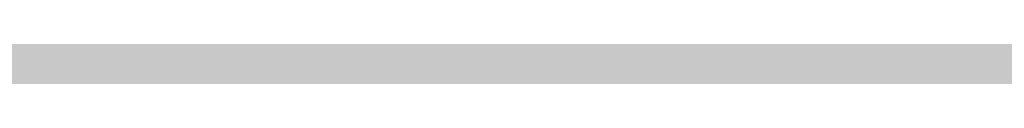
# Model space of a CAD drawing. Units: millimetres. Extents: x -22994 to 29398, y -19990 to 20176.
# Tile 98 of 135: x 229.428 to 230.597, y 84.585 to 84.615. Entities that reach past the tile are written whole.
import ezdxf
from ezdxf import colors
from ezdxf.entities.mleader import LeaderData, LeaderLine
from ezdxf.math import Vec2, Vec3

# ---------------------------------------------------------------- set-up
doc = ezdxf.new("R2010")
doc.units = ezdxf.units.MM
doc.header["$MEASUREMENT"] = 0
doc.layers.add('M-ANNO-TEXT', color=7, linetype='Continuous', lineweight=25)
doc.layers.add('M-DIMS', color=2, linetype='Continuous', lineweight=18)
doc.styles.get("Standard").update_dxf_attribs({"font": 'arial.ttf'})
doc.dimstyles.get("Standard").update_dxf_attribs({"dimtxt": 0.18, "dimasz": 10000, "dimexe": 0.18, "dimexo": 0.0625, "dimgap": 0.09, "dimtad": 0, "dimtih": 1, "dimtoh": 1, "dimdec": 0, "dimzin": 0, "dimdsep": 46, "dimtxsty": 'Standard', "dimcen": 0.09, "dimadec": 0, "dimazin": 0, "dimtfac": 1, "dimtdec": 0, "dimtofl": 0, "dimtmove": 0, "dimatfit": 3, "dimfxl": 1, "dimtolj": 1, "dimtzin": 0, "dimlwd": 30, "dimarcsym": 0})

# ---------------------------------------------------------------- blocks, each defined once
blk = doc.blocks.new('*D2')
at = {"layer": 'Defpoints', "color": 0, "transparency": 16777216}
for p in [(6.6773, 10.2713), (290.852, 10.2713), (290.852, -5.0787)]:
    blk.add_point(p, dxfattribs=at)
at = {"layer": 'M-DIMS', "color": 0, "lineweight": -2, "transparency": 16777216}
for p, q in [((6.6773, 10.2088), (6.6773, -5.2587)), ((290.852, 10.2088), (290.852, -5.2587))]:
    blk.add_line(p, q, dxfattribs=at)
at = {"layer": 'M-DIMS', "color": 0, "lineweight": 30, "transparency": 16777216}
for p, q in [((-9993.3227, -5.0787), (-19993.3227, -5.0787)), ((10290.852, -5.0787), (20290.852, -5.0787))]:
    blk.add_line(p, q, dxfattribs=at)
at = {"layer": 'M-DIMS', "color": 0, "transparency": 16777216}
for points in [[(-9993.3227, 1661.5879), (-9993.3227, -1671.7454), (6.6773, -5.0787)], [(10290.852, 1661.5879), (10290.852, -1671.7454), (290.852, -5.0787)]]:
    blk.add_solid(points, dxfattribs=at)
at = {"layer": 'M-DIMS', "color": 0, "transparency": 16777216, "insert": (148.7647, -5.0787), "char_height": 0.18, "attachment_point": 5}
blk.add_mtext('\\A1;284.2', dxfattribs=at)
blk = doc.blocks.new('*D3')
at = {"layer": 'Defpoints', "color": 0, "transparency": 16777216}
for p in [(110.2647, 204.1654), (110.2647, 176.3662), (95.8327, 127.967)]:
    blk.add_point(p, dxfattribs=at)
at = {"layer": 'M-DIMS', "color": 0, "lineweight": -2, "transparency": 16777216}
for p, q in [((95.8327, 128.0295), (95.8327, 204.3454)), ((110.2647, 176.4287), (110.2647, 204.3454))]:
    blk.add_line(p, q, dxfattribs=at)
at = {"layer": 'M-DIMS', "color": 0, "lineweight": 30, "transparency": 16777216}
for p, q in [((-9904.1673, 204.1654), (-19904.1673, 204.1654)), ((10110.2647, 204.1654), (20110.2647, 204.1654))]:
    blk.add_line(p, q, dxfattribs=at)
at = {"layer": 'M-DIMS', "color": 0, "transparency": 16777216}
for points in [[(-9904.1673, 1870.8321), (-9904.1673, -1462.5013), (95.8327, 204.1654)], [(10110.2647, 1870.8321), (10110.2647, -1462.5013), (110.2647, 204.1654)]]:
    blk.add_solid(points, dxfattribs=at)
at = {"layer": 'M-DIMS', "color": 0, "transparency": 16777216, "insert": (103.0487, 204.1654), "char_height": 0.18, "attachment_point": 5}
blk.add_mtext('\\A1;14.432', dxfattribs=at)
blk = doc.blocks.new('*D4')
at = {"layer": 'Defpoints', "color": 0, "transparency": 16777216}
for p in [(116.2647, 204.1654), (110.2647, 176.3662), (116.2647, 176.3662)]:
    blk.add_point(p, dxfattribs=at)
at = {"layer": 'M-DIMS', "color": 0, "lineweight": -2, "transparency": 16777216}
for p, q in [((110.2647, 176.4287), (110.2647, 204.3454)), ((116.2647, 176.4287), (116.2647, 204.3454))]:
    blk.add_line(p, q, dxfattribs=at)
at = {"layer": 'M-DIMS', "color": 0, "lineweight": 30, "transparency": 16777216}
for p, q in [((-9889.7353, 204.1654), (-19889.7353, 204.1654)), ((10116.2647, 204.1654), (20116.2647, 204.1654))]:
    blk.add_line(p, q, dxfattribs=at)
at = {"layer": 'M-DIMS', "color": 0, "transparency": 16777216}
for points in [[(-9889.7353, 1870.8321), (-9889.7353, -1462.5013), (110.2647, 204.1654)], [(10116.2647, 1870.8321), (10116.2647, -1462.5013), (116.2647, 204.1654)]]:
    blk.add_solid(points, dxfattribs=at)
at = {"layer": 'M-DIMS', "color": 0, "transparency": 16777216, "insert": (113.2647, 204.1654), "char_height": 0.18, "attachment_point": 5}
blk.add_mtext('\\A1;6', dxfattribs=at)
blk = doc.blocks.new('*D5')
at = {"layer": 'Defpoints', "color": 0, "transparency": 16777216}
for p in [(181.2647, 204.1654), (116.2647, 176.3662), (181.2647, 176.3662)]:
    blk.add_point(p, dxfattribs=at)
at = {"layer": 'M-DIMS', "color": 0, "lineweight": -2, "transparency": 16777216}
for p, q in [((116.2647, 176.4287), (116.2647, 204.3454)), ((181.2647, 176.4287), (181.2647, 204.3454))]:
    blk.add_line(p, q, dxfattribs=at)
at = {"layer": 'M-DIMS', "color": 0, "lineweight": 30, "transparency": 16777216}
for p, q in [((-9883.7353, 204.1654), (-19883.7353, 204.1654)), ((10181.2647, 204.1654), (20181.2647, 204.1654))]:
    blk.add_line(p, q, dxfattribs=at)
at = {"layer": 'M-DIMS', "color": 0, "transparency": 16777216}
for points in [[(-9883.7353, 1870.8321), (-9883.7353, -1462.5013), (116.2647, 204.1654)], [(10181.2647, 1870.8321), (10181.2647, -1462.5013), (181.2647, 204.1654)]]:
    blk.add_solid(points, dxfattribs=at)
at = {"layer": 'M-DIMS', "color": 0, "transparency": 16777216, "insert": (148.7647, 204.1654), "char_height": 0.18, "attachment_point": 5}
blk.add_mtext('\\A1;65', dxfattribs=at)
blk = doc.blocks.new('*D6')
at = {"layer": 'Defpoints', "color": 0, "transparency": 16777216}
for p in [(187.2647, 204.1654), (181.2647, 176.3662), (187.2647, 176.3662)]:
    blk.add_point(p, dxfattribs=at)
at = {"layer": 'M-DIMS', "color": 0, "lineweight": -2, "transparency": 16777216}
for p, q in [((181.2647, 176.4287), (181.2647, 204.3454)), ((187.2647, 176.4287), (187.2647, 204.3454))]:
    blk.add_line(p, q, dxfattribs=at)
at = {"layer": 'M-DIMS', "color": 0, "lineweight": 30, "transparency": 16777216}
for p, q in [((-9818.7353, 204.1654), (-19818.7353, 204.1654)), ((10187.2647, 204.1654), (20187.2647, 204.1654))]:
    blk.add_line(p, q, dxfattribs=at)
at = {"layer": 'M-DIMS', "color": 0, "transparency": 16777216}
for points in [[(-9818.7353, 1870.8321), (-9818.7353, -1462.5013), (181.2647, 204.1654)], [(10187.2647, 1870.8321), (10187.2647, -1462.5013), (187.2647, 204.1654)]]:
    blk.add_solid(points, dxfattribs=at)
at = {"layer": 'M-DIMS', "color": 0, "transparency": 16777216, "insert": (184.2647, 204.1654), "char_height": 0.18, "attachment_point": 5}
blk.add_mtext('\\A1;6', dxfattribs=at)
blk = doc.blocks.new('*D7')
at = {"layer": 'Defpoints', "color": 0, "transparency": 16777216}
for p in [(201.6967, 204.1654), (187.2647, 176.3662), (201.6967, 127.967)]:
    blk.add_point(p, dxfattribs=at)
at = {"layer": 'M-DIMS', "color": 0, "lineweight": -2, "transparency": 16777216}
for p, q in [((187.2647, 176.4287), (187.2647, 204.3454)), ((201.6967, 128.0295), (201.6967, 204.3454))]:
    blk.add_line(p, q, dxfattribs=at)
at = {"layer": 'M-DIMS', "color": 0, "lineweight": 30, "transparency": 16777216}
for p, q in [((-9812.7353, 204.1654), (-19812.7353, 204.1654)), ((10201.6967, 204.1654), (20201.6967, 204.1654))]:
    blk.add_line(p, q, dxfattribs=at)
at = {"layer": 'M-DIMS', "color": 0, "transparency": 16777216}
for points in [[(-9812.7353, 1870.8321), (-9812.7353, -1462.5013), (187.2647, 204.1654)], [(10201.6967, 1870.8321), (10201.6967, -1462.5013), (201.6967, 204.1654)]]:
    blk.add_solid(points, dxfattribs=at)
at = {"layer": 'M-DIMS', "color": 0, "transparency": 16777216, "insert": (194.4807, 204.1654), "char_height": 0.18, "attachment_point": 5}
blk.add_mtext('\\A1;14.432', dxfattribs=at)
blk = doc.blocks.new('*D8')
at = {"layer": 'Defpoints', "color": 0, "transparency": 16777216}
for p in [(227.6485, 204.1654), (227.6485, 146.7296), (201.6967, 127.967)]:
    blk.add_point(p, dxfattribs=at)
at = {"layer": 'M-DIMS', "color": 0, "lineweight": -2, "transparency": 16777216}
for p, q in [((201.6967, 128.0295), (201.6967, 204.3454)), ((227.6485, 146.7921), (227.6485, 204.3454))]:
    blk.add_line(p, q, dxfattribs=at)
at = {"layer": 'M-DIMS', "color": 0, "lineweight": 30, "transparency": 16777216}
for p, q in [((-9798.3033, 204.1654), (-19798.3033, 204.1654)), ((10227.6485, 204.1654), (20227.6485, 204.1654))]:
    blk.add_line(p, q, dxfattribs=at)
at = {"layer": 'M-DIMS', "color": 0, "transparency": 16777216}
for points in [[(-9798.3033, 1870.8321), (-9798.3033, -1462.5013), (201.6967, 204.1654)], [(10227.6485, 1870.8321), (10227.6485, -1462.5013), (227.6485, 204.1654)]]:
    blk.add_solid(points, dxfattribs=at)
at = {"layer": 'M-DIMS', "color": 0, "transparency": 16777216, "insert": (214.6726, 204.1654), "char_height": 0.18, "attachment_point": 5}
blk.add_mtext('\\A1;25.95', dxfattribs=at)
blk = doc.blocks.new('*D9')
at = {"layer": 'Defpoints', "color": 0, "transparency": 16777216}
for p in [(187.2647, 176.3662), (306.202, 176.3662), (290.852, 10.2713)]:
    blk.add_point(p, dxfattribs=at)
at = {"layer": 'M-DIMS', "color": 0, "lineweight": 30, "transparency": 16777216}
for p, q in [((306.202, 10176.3662), (306.202, 20176.3662)), ((306.202, -9989.7287), (306.202, -19989.7287))]:
    blk.add_line(p, q, dxfattribs=at)
at = {"layer": 'M-DIMS', "color": 0, "lineweight": -2, "transparency": 16777216}
for p, q in [((187.3272, 176.3662), (306.382, 176.3662)), ((290.9145, 10.2713), (306.382, 10.2713))]:
    blk.add_line(p, q, dxfattribs=at)
at = {"layer": 'M-DIMS', "color": 0, "transparency": 16777216}
for points in [[(-1360.4646, 10176.3662), (1972.8687, 10176.3662), (306.202, 176.3662)], [(-1360.4646, -9989.7287), (1972.8687, -9989.7287), (306.202, 10.2713)]]:
    blk.add_solid(points, dxfattribs=at)
at = {"layer": 'M-DIMS', "color": 0, "transparency": 16777216, "insert": (306.202, 93.3187), "char_height": 0.18, "attachment_point": 5}
blk.add_mtext('\\A1;166.1', dxfattribs=at)
blk = doc.blocks.new('*D10')
at = {"layer": 'Defpoints', "color": 0, "transparency": 16777216}
for p in [(125.6498, 136.0713), (133.3459, 136.0713), (133.3459, -5.0787)]:
    blk.add_point(p, dxfattribs=at)
at = {"layer": 'M-DIMS', "color": 0, "lineweight": -2, "transparency": 16777216}
for p, q in [((125.6498, 136.0088), (125.6498, -5.2587)), ((133.3459, 136.0088), (133.3459, -5.2587))]:
    blk.add_line(p, q, dxfattribs=at)
at = {"layer": 'M-DIMS', "color": 0, "lineweight": 30, "transparency": 16777216}
for p, q in [((-9874.3502, -5.0787), (-19874.3502, -5.0787)), ((10133.3459, -5.0787), (20133.3459, -5.0787))]:
    blk.add_line(p, q, dxfattribs=at)
at = {"layer": 'M-DIMS', "color": 0, "transparency": 16777216}
for points in [[(-9874.3502, 1661.5879), (-9874.3502, -1671.7454), (125.6498, -5.0787)], [(10133.3459, 1661.5879), (10133.3459, -1671.7454), (133.3459, -5.0787)]]:
    blk.add_solid(points, dxfattribs=at)
at = {"layer": 'M-DIMS', "color": 0, "transparency": 16777216, "insert": (129.4978, -5.0787), "char_height": 0.18, "attachment_point": 5}
blk.add_mtext('\\A1;7.696', dxfattribs=at)
blk = doc.blocks.new('*D11')
at = {"layer": 'Defpoints', "color": 0, "transparency": 16777216}
for p in [(133.3459, 136.0713), (135.6498, 136.0713), (135.6498, -5.0787)]:
    blk.add_point(p, dxfattribs=at)
at = {"layer": 'M-DIMS', "color": 0, "lineweight": -2, "transparency": 16777216}
for p, q in [((133.3459, 136.0088), (133.3459, -5.2587)), ((135.6498, 136.0088), (135.6498, -5.2587))]:
    blk.add_line(p, q, dxfattribs=at)
at = {"layer": 'M-DIMS', "color": 0, "lineweight": 30, "transparency": 16777216}
for p, q in [((-9866.6541, -5.0787), (-19866.6541, -5.0787)), ((10135.6498, -5.0787), (20135.6498, -5.0787))]:
    blk.add_line(p, q, dxfattribs=at)
at = {"layer": 'M-DIMS', "color": 0, "transparency": 16777216}
for points in [[(-9866.6541, 1661.5879), (-9866.6541, -1671.7454), (133.3459, -5.0787)], [(10135.6498, 1661.5879), (10135.6498, -1671.7454), (135.6498, -5.0787)]]:
    blk.add_solid(points, dxfattribs=at)
at = {"layer": 'M-DIMS', "color": 0, "transparency": 16777216, "insert": (134.4978, -5.0787), "char_height": 0.18, "attachment_point": 5}
blk.add_mtext('\\A1;2.304', dxfattribs=at)
blk = doc.blocks.new('*D12')
at = {"layer": 'Defpoints', "color": 0, "transparency": 16777216}
for p in [(135.6498, 136.0713), (145.6498, 136.0713), (145.6498, -5.0787)]:
    blk.add_point(p, dxfattribs=at)
at = {"layer": 'M-DIMS', "color": 0, "lineweight": -2, "transparency": 16777216}
for p, q in [((135.6498, 136.0088), (135.6498, -5.2587)), ((145.6498, 136.0088), (145.6498, -5.2587))]:
    blk.add_line(p, q, dxfattribs=at)
at = {"layer": 'M-DIMS', "color": 0, "lineweight": 30, "transparency": 16777216}
for p, q in [((-9864.3502, -5.0787), (-19864.3502, -5.0787)), ((10145.6498, -5.0787), (20145.6498, -5.0787))]:
    blk.add_line(p, q, dxfattribs=at)
at = {"layer": 'M-DIMS', "color": 0, "transparency": 16777216}
for points in [[(-9864.3502, 1661.5879), (-9864.3502, -1671.7454), (135.6498, -5.0787)], [(10145.6498, 1661.5879), (10145.6498, -1671.7454), (145.6498, -5.0787)]]:
    blk.add_solid(points, dxfattribs=at)
at = {"layer": 'M-DIMS', "color": 0, "transparency": 16777216, "insert": (140.6498, -5.0787), "char_height": 0.18, "attachment_point": 5}
blk.add_mtext('\\A1;10', dxfattribs=at)
blk = doc.blocks.new('*D13')
at = {"layer": 'Defpoints', "color": 0, "transparency": 16777216}
for p in [(145.6498, 136.0713), (155.6498, 136.0713), (155.6498, -5.0787)]:
    blk.add_point(p, dxfattribs=at)
at = {"layer": 'M-DIMS', "color": 0, "lineweight": -2, "transparency": 16777216}
for p, q in [((145.6498, 136.0088), (145.6498, -5.2587)), ((155.6498, 136.0088), (155.6498, -5.2587))]:
    blk.add_line(p, q, dxfattribs=at)
at = {"layer": 'M-DIMS', "color": 0, "lineweight": 30, "transparency": 16777216}
for p, q in [((-9854.3502, -5.0787), (-19854.3502, -5.0787)), ((10155.6498, -5.0787), (20155.6498, -5.0787))]:
    blk.add_line(p, q, dxfattribs=at)
at = {"layer": 'M-DIMS', "color": 0, "transparency": 16777216}
for points in [[(-9854.3502, 1661.5879), (-9854.3502, -1671.7454), (145.6498, -5.0787)], [(10155.6498, 1661.5879), (10155.6498, -1671.7454), (155.6498, -5.0787)]]:
    blk.add_solid(points, dxfattribs=at)
at = {"layer": 'M-DIMS', "color": 0, "transparency": 16777216, "insert": (150.6498, -5.0787), "char_height": 0.18, "attachment_point": 5}
blk.add_mtext('\\A1;10', dxfattribs=at)
blk = doc.blocks.new('*D14')
at = {"layer": 'Defpoints', "color": 0, "transparency": 16777216}
for p in [(155.6498, 136.0713), (165.6498, 136.0713), (165.6498, -5.0787)]:
    blk.add_point(p, dxfattribs=at)
at = {"layer": 'M-DIMS', "color": 0, "lineweight": -2, "transparency": 16777216}
for p, q in [((155.6498, 136.0088), (155.6498, -5.2587)), ((165.6498, 136.0088), (165.6498, -5.2587))]:
    blk.add_line(p, q, dxfattribs=at)
at = {"layer": 'M-DIMS', "color": 0, "lineweight": 30, "transparency": 16777216}
for p, q in [((-9844.3502, -5.0787), (-19844.3502, -5.0787)), ((10165.6498, -5.0787), (20165.6498, -5.0787))]:
    blk.add_line(p, q, dxfattribs=at)
at = {"layer": 'M-DIMS', "color": 0, "transparency": 16777216}
for points in [[(-9844.3502, 1661.5879), (-9844.3502, -1671.7454), (155.6498, -5.0787)], [(10165.6498, 1661.5879), (10165.6498, -1671.7454), (165.6498, -5.0787)]]:
    blk.add_solid(points, dxfattribs=at)
at = {"layer": 'M-DIMS', "color": 0, "transparency": 16777216, "insert": (160.6498, -5.0787), "char_height": 0.18, "attachment_point": 5}
blk.add_mtext('\\A1;10', dxfattribs=at)
blk = doc.blocks.new('*D15')
at = {"layer": 'Defpoints', "color": 0, "transparency": 16777216}
for p in [(173.3459, 154.788), (173.3459, 136.0713), (306.202, 136.0713)]:
    blk.add_point(p, dxfattribs=at)
at = {"layer": 'M-DIMS', "color": 0, "lineweight": 30, "transparency": 16777216}
for p, q in [((306.202, 10154.788), (306.202, 20154.788)), ((306.202, -9863.9287), (306.202, -19863.9287))]:
    blk.add_line(p, q, dxfattribs=at)
at = {"layer": 'M-DIMS', "color": 0, "lineweight": -2, "transparency": 16777216}
for p, q in [((173.4084, 154.788), (306.382, 154.788)), ((173.4084, 136.0713), (306.382, 136.0713))]:
    blk.add_line(p, q, dxfattribs=at)
at = {"layer": 'M-DIMS', "color": 0, "transparency": 16777216}
for points in [[(-1360.4646, 10154.788), (1972.8687, 10154.788), (306.202, 154.788)], [(-1360.4646, -9863.9287), (1972.8687, -9863.9287), (306.202, 136.0713)]]:
    blk.add_solid(points, dxfattribs=at)
at = {"layer": 'M-DIMS', "color": 0, "transparency": 16777216, "insert": (306.202, 145.4297), "char_height": 0.18, "attachment_point": 5}
blk.add_mtext('\\A1;18.717', dxfattribs=at)
blk = doc.blocks.new('*D16')
at = {"layer": 'Defpoints', "color": 0, "transparency": 16777216}
for p in [(120.1702, 204.1654), (110.4658, 48.0349), (120.1702, 48.0349)]:
    blk.add_point(p, dxfattribs=at)
at = {"layer": 'M-DIMS', "color": 0, "lineweight": -2, "transparency": 16777216}
for p, q in [((110.4658, 48.0974), (110.4658, 204.3454)), ((120.1702, 48.0974), (120.1702, 204.3454))]:
    blk.add_line(p, q, dxfattribs=at)
at = {"layer": 'M-DIMS', "color": 0, "lineweight": 30, "transparency": 16777216}
for p, q in [((-9889.5342, 204.1654), (-19889.5342, 204.1654)), ((10120.1702, 204.1654), (20120.1702, 204.1654))]:
    blk.add_line(p, q, dxfattribs=at)
at = {"layer": 'M-DIMS', "color": 0, "transparency": 16777216}
for points in [[(-9889.5342, 1870.8321), (-9889.5342, -1462.5013), (110.4658, 204.1654)], [(10120.1702, 1870.8321), (10120.1702, -1462.5013), (120.1702, 204.1654)]]:
    blk.add_solid(points, dxfattribs=at)
at = {"layer": 'M-DIMS', "color": 0, "transparency": 16777216, "insert": (115.318, 204.1654), "char_height": 0.18, "attachment_point": 5}
blk.add_mtext('\\A1;9.704', dxfattribs=at)
blk = doc.blocks.new('*D17')
at = {"layer": 'Defpoints', "color": 0, "transparency": 16777216}
for p in [(126.1702, 204.1654), (120.1702, 48.0349), (126.1702, 48.0349)]:
    blk.add_point(p, dxfattribs=at)
at = {"layer": 'M-DIMS', "color": 0, "lineweight": -2, "transparency": 16777216}
for p, q in [((120.1702, 48.0974), (120.1702, 204.3454)), ((126.1702, 48.0974), (126.1702, 204.3454))]:
    blk.add_line(p, q, dxfattribs=at)
at = {"layer": 'M-DIMS', "color": 0, "lineweight": 30, "transparency": 16777216}
for p, q in [((-9879.8298, 204.1654), (-19879.8298, 204.1654)), ((10126.1702, 204.1654), (20126.1702, 204.1654))]:
    blk.add_line(p, q, dxfattribs=at)
at = {"layer": 'M-DIMS', "color": 0, "transparency": 16777216}
for points in [[(-9879.8298, 1870.8321), (-9879.8298, -1462.5013), (120.1702, 204.1654)], [(10126.1702, 1870.8321), (10126.1702, -1462.5013), (126.1702, 204.1654)]]:
    blk.add_solid(points, dxfattribs=at)
at = {"layer": 'M-DIMS', "color": 0, "transparency": 16777216, "insert": (123.1702, 204.1654), "char_height": 0.18, "attachment_point": 5}
blk.add_mtext('\\A1;6', dxfattribs=at)
blk = doc.blocks.new('*D18')
at = {"layer": 'Defpoints', "color": 0, "transparency": 16777216}
for p in [(132.1702, 204.1654), (126.1702, 48.0349), (132.1702, 48.0349)]:
    blk.add_point(p, dxfattribs=at)
at = {"layer": 'M-DIMS', "color": 0, "lineweight": -2, "transparency": 16777216}
for p, q in [((126.1702, 48.0974), (126.1702, 204.3454)), ((132.1702, 48.0974), (132.1702, 204.3454))]:
    blk.add_line(p, q, dxfattribs=at)
at = {"layer": 'M-DIMS', "color": 0, "lineweight": 30, "transparency": 16777216}
for p, q in [((-9873.8298, 204.1654), (-19873.8298, 204.1654)), ((10132.1702, 204.1654), (20132.1702, 204.1654))]:
    blk.add_line(p, q, dxfattribs=at)
at = {"layer": 'M-DIMS', "color": 0, "transparency": 16777216}
for points in [[(-9873.8298, 1870.8321), (-9873.8298, -1462.5013), (126.1702, 204.1654)], [(10132.1702, 1870.8321), (10132.1702, -1462.5013), (132.1702, 204.1654)]]:
    blk.add_solid(points, dxfattribs=at)
at = {"layer": 'M-DIMS', "color": 0, "transparency": 16777216, "insert": (129.1702, 204.1654), "char_height": 0.18, "attachment_point": 5}
blk.add_mtext('\\A1;6', dxfattribs=at)
blk = doc.blocks.new('*D19')
at = {"layer": 'Defpoints', "color": 0, "transparency": 16777216}
for p in [(138.1702, 204.1654), (132.1702, 48.0349), (138.1702, 48.0349)]:
    blk.add_point(p, dxfattribs=at)
at = {"layer": 'M-DIMS', "color": 0, "lineweight": -2, "transparency": 16777216}
for p, q in [((132.1702, 48.0974), (132.1702, 204.3454)), ((138.1702, 48.0974), (138.1702, 204.3454))]:
    blk.add_line(p, q, dxfattribs=at)
at = {"layer": 'M-DIMS', "color": 0, "lineweight": 30, "transparency": 16777216}
for p, q in [((-9867.8298, 204.1654), (-19867.8298, 204.1654)), ((10138.1702, 204.1654), (20138.1702, 204.1654))]:
    blk.add_line(p, q, dxfattribs=at)
at = {"layer": 'M-DIMS', "color": 0, "transparency": 16777216}
for points in [[(-9867.8298, 1870.8321), (-9867.8298, -1462.5013), (132.1702, 204.1654)], [(10138.1702, 1870.8321), (10138.1702, -1462.5013), (138.1702, 204.1654)]]:
    blk.add_solid(points, dxfattribs=at)
at = {"layer": 'M-DIMS', "color": 0, "transparency": 16777216, "insert": (135.1702, 204.1654), "char_height": 0.18, "attachment_point": 5}
blk.add_mtext('\\A1;6', dxfattribs=at)
blk = doc.blocks.new('*D20')
at = {"layer": 'Defpoints', "color": 0, "transparency": 16777216}
for p in [(144.1702, 204.1654), (138.1702, 48.0349), (144.1702, 48.0349)]:
    blk.add_point(p, dxfattribs=at)
at = {"layer": 'M-DIMS', "color": 0, "lineweight": -2, "transparency": 16777216}
for p, q in [((138.1702, 48.0974), (138.1702, 204.3454)), ((144.1702, 48.0974), (144.1702, 204.3454))]:
    blk.add_line(p, q, dxfattribs=at)
at = {"layer": 'M-DIMS', "color": 0, "lineweight": 30, "transparency": 16777216}
for p, q in [((-9861.8298, 204.1654), (-19861.8298, 204.1654)), ((10144.1702, 204.1654), (20144.1702, 204.1654))]:
    blk.add_line(p, q, dxfattribs=at)
at = {"layer": 'M-DIMS', "color": 0, "transparency": 16777216}
for points in [[(-9861.8298, 1870.8321), (-9861.8298, -1462.5013), (138.1702, 204.1654)], [(10144.1702, 1870.8321), (10144.1702, -1462.5013), (144.1702, 204.1654)]]:
    blk.add_solid(points, dxfattribs=at)
at = {"layer": 'M-DIMS', "color": 0, "transparency": 16777216, "insert": (141.1702, 204.1654), "char_height": 0.18, "attachment_point": 5}
blk.add_mtext('\\A1;6', dxfattribs=at)
blk = doc.blocks.new('*D21')
at = {"layer": 'Defpoints', "color": 0, "transparency": 16777216}
for p in [(149.1157, 204.1654), (144.1702, 48.0349), (149.1157, 48.0349)]:
    blk.add_point(p, dxfattribs=at)
at = {"layer": 'M-DIMS', "color": 0, "lineweight": -2, "transparency": 16777216}
for p, q in [((144.1702, 48.0974), (144.1702, 204.3454)), ((149.1157, 48.0974), (149.1157, 204.3454))]:
    blk.add_line(p, q, dxfattribs=at)
at = {"layer": 'M-DIMS', "color": 0, "lineweight": 30, "transparency": 16777216}
for p, q in [((-9855.8298, 204.1654), (-19855.8298, 204.1654)), ((10149.1157, 204.1654), (20149.1157, 204.1654))]:
    blk.add_line(p, q, dxfattribs=at)
at = {"layer": 'M-DIMS', "color": 0, "transparency": 16777216}
for points in [[(-9855.8298, 1870.8321), (-9855.8298, -1462.5013), (144.1702, 204.1654)], [(10149.1157, 1870.8321), (10149.1157, -1462.5013), (149.1157, 204.1654)]]:
    blk.add_solid(points, dxfattribs=at)
at = {"layer": 'M-DIMS', "color": 0, "transparency": 16777216, "insert": (146.6429, 204.1654), "char_height": 0.18, "attachment_point": 5}
blk.add_mtext('\\A1;4.945', dxfattribs=at)
blk = doc.blocks.new('*D22')
at = {"layer": 'Defpoints', "color": 0, "transparency": 16777216}
for p in [(149.1157, 30.9895), (155.1157, 30.9895), (155.1157, -5.0787)]:
    blk.add_point(p, dxfattribs=at)
at = {"layer": 'M-DIMS', "color": 0, "lineweight": -2, "transparency": 16777216}
for p, q in [((149.1157, 30.927), (149.1157, -5.2587)), ((155.1157, 30.927), (155.1157, -5.2587))]:
    blk.add_line(p, q, dxfattribs=at)
at = {"layer": 'M-DIMS', "color": 0, "lineweight": 30, "transparency": 16777216}
for p, q in [((-9850.8843, -5.0787), (-19850.8843, -5.0787)), ((10155.1157, -5.0787), (20155.1157, -5.0787))]:
    blk.add_line(p, q, dxfattribs=at)
at = {"layer": 'M-DIMS', "color": 0, "transparency": 16777216}
for points in [[(-9850.8843, 1661.5879), (-9850.8843, -1671.7454), (149.1157, -5.0787)], [(10155.1157, 1661.5879), (10155.1157, -1671.7454), (155.1157, -5.0787)]]:
    blk.add_solid(points, dxfattribs=at)
at = {"layer": 'M-DIMS', "color": 0, "transparency": 16777216, "insert": (152.1157, -5.0787), "char_height": 0.18, "attachment_point": 5}
blk.add_mtext('\\A1;6', dxfattribs=at)
blk = doc.blocks.new('*D23')
at = {"layer": 'Defpoints', "color": 0, "transparency": 16777216}
for p in [(155.1157, 30.9895), (161.1157, 30.9895), (161.1157, -5.0787)]:
    blk.add_point(p, dxfattribs=at)
at = {"layer": 'M-DIMS', "color": 0, "lineweight": -2, "transparency": 16777216}
for p, q in [((155.1157, 30.927), (155.1157, -5.2587)), ((161.1157, 30.927), (161.1157, -5.2587))]:
    blk.add_line(p, q, dxfattribs=at)
at = {"layer": 'M-DIMS', "color": 0, "lineweight": 30, "transparency": 16777216}
for p, q in [((-9844.8843, -5.0787), (-19844.8843, -5.0787)), ((10161.1157, -5.0787), (20161.1157, -5.0787))]:
    blk.add_line(p, q, dxfattribs=at)
at = {"layer": 'M-DIMS', "color": 0, "transparency": 16777216}
for points in [[(-9844.8843, 1661.5879), (-9844.8843, -1671.7454), (155.1157, -5.0787)], [(10161.1157, 1661.5879), (10161.1157, -1671.7454), (161.1157, -5.0787)]]:
    blk.add_solid(points, dxfattribs=at)
at = {"layer": 'M-DIMS', "color": 0, "transparency": 16777216, "insert": (158.1157, -5.0787), "char_height": 0.18, "attachment_point": 5}
blk.add_mtext('\\A1;6', dxfattribs=at)
blk = doc.blocks.new('*D24')
at = {"layer": 'Defpoints', "color": 0, "transparency": 16777216}
for p in [(161.1157, 30.9895), (166.4387, 30.9895), (166.4387, -5.0787)]:
    blk.add_point(p, dxfattribs=at)
at = {"layer": 'M-DIMS', "color": 0, "lineweight": -2, "transparency": 16777216}
for p, q in [((161.1157, 30.927), (161.1157, -5.2587)), ((166.4387, 30.927), (166.4387, -5.2587))]:
    blk.add_line(p, q, dxfattribs=at)
at = {"layer": 'M-DIMS', "color": 0, "lineweight": 30, "transparency": 16777216}
for p, q in [((-9838.8843, -5.0787), (-19838.8843, -5.0787)), ((10166.4387, -5.0787), (20166.4387, -5.0787))]:
    blk.add_line(p, q, dxfattribs=at)
at = {"layer": 'M-DIMS', "color": 0, "transparency": 16777216}
for points in [[(-9838.8843, 1661.5879), (-9838.8843, -1671.7454), (161.1157, -5.0787)], [(10166.4387, 1661.5879), (10166.4387, -1671.7454), (166.4387, -5.0787)]]:
    blk.add_solid(points, dxfattribs=at)
at = {"layer": 'M-DIMS', "color": 0, "transparency": 16777216, "insert": (163.7772, -5.0787), "char_height": 0.18, "attachment_point": 5}
blk.add_mtext('\\A1;5.323', dxfattribs=at)
blk = doc.blocks.new('*D25')
at = {"layer": 'Defpoints', "color": 0, "transparency": 16777216}
for p in [(166.4387, 30.9895), (172.4387, 30.9895), (172.4387, -5.0787)]:
    blk.add_point(p, dxfattribs=at)
at = {"layer": 'M-DIMS', "color": 0, "lineweight": -2, "transparency": 16777216}
for p, q in [((166.4387, 30.927), (166.4387, -5.2587)), ((172.4387, 30.927), (172.4387, -5.2587))]:
    blk.add_line(p, q, dxfattribs=at)
at = {"layer": 'M-DIMS', "color": 0, "lineweight": 30, "transparency": 16777216}
for p, q in [((-9833.5613, -5.0787), (-19833.5613, -5.0787)), ((10172.4387, -5.0787), (20172.4387, -5.0787))]:
    blk.add_line(p, q, dxfattribs=at)
at = {"layer": 'M-DIMS', "color": 0, "transparency": 16777216}
for points in [[(-9833.5613, 1661.5879), (-9833.5613, -1671.7454), (166.4387, -5.0787)], [(10172.4387, 1661.5879), (10172.4387, -1671.7454), (172.4387, -5.0787)]]:
    blk.add_solid(points, dxfattribs=at)
at = {"layer": 'M-DIMS', "color": 0, "transparency": 16777216, "insert": (169.4387, -5.0787), "char_height": 0.18, "attachment_point": 5}
blk.add_mtext('\\A1;6', dxfattribs=at)
blk = doc.blocks.new('*D26')
at = {"layer": 'Defpoints', "color": 0, "transparency": 16777216}
for p in [(172.4387, 30.9895), (178.4387, 30.9895), (178.4387, -5.0787)]:
    blk.add_point(p, dxfattribs=at)
at = {"layer": 'M-DIMS', "color": 0, "lineweight": -2, "transparency": 16777216}
for p, q in [((172.4387, 30.927), (172.4387, -5.2587)), ((178.4387, 30.927), (178.4387, -5.2587))]:
    blk.add_line(p, q, dxfattribs=at)
at = {"layer": 'M-DIMS', "color": 0, "lineweight": 30, "transparency": 16777216}
for p, q in [((-9827.5613, -5.0787), (-19827.5613, -5.0787)), ((10178.4387, -5.0787), (20178.4387, -5.0787))]:
    blk.add_line(p, q, dxfattribs=at)
at = {"layer": 'M-DIMS', "color": 0, "transparency": 16777216}
for points in [[(-9827.5613, 1661.5879), (-9827.5613, -1671.7454), (172.4387, -5.0787)], [(10178.4387, 1661.5879), (10178.4387, -1671.7454), (178.4387, -5.0787)]]:
    blk.add_solid(points, dxfattribs=at)
at = {"layer": 'M-DIMS', "color": 0, "transparency": 16777216, "insert": (175.4387, -5.0787), "char_height": 0.18, "attachment_point": 5}
blk.add_mtext('\\A1;6', dxfattribs=at)
blk = doc.blocks.new('*D27')
at = {"layer": 'Defpoints', "color": 0, "transparency": 16777216}
for p in [(178.4387, 30.9895), (188.1175, 30.9895), (188.1175, -5.0787)]:
    blk.add_point(p, dxfattribs=at)
at = {"layer": 'M-DIMS', "color": 0, "lineweight": -2, "transparency": 16777216}
for p, q in [((178.4387, 30.927), (178.4387, -5.2587)), ((188.1175, 30.927), (188.1175, -5.2587))]:
    blk.add_line(p, q, dxfattribs=at)
at = {"layer": 'M-DIMS', "color": 0, "lineweight": 30, "transparency": 16777216}
for p, q in [((-9821.5613, -5.0787), (-19821.5613, -5.0787)), ((10188.1175, -5.0787), (20188.1175, -5.0787))]:
    blk.add_line(p, q, dxfattribs=at)
at = {"layer": 'M-DIMS', "color": 0, "transparency": 16777216}
for points in [[(-9821.5613, 1661.5879), (-9821.5613, -1671.7454), (178.4387, -5.0787)], [(10188.1175, 1661.5879), (10188.1175, -1671.7454), (188.1175, -5.0787)]]:
    blk.add_solid(points, dxfattribs=at)
at = {"layer": 'M-DIMS', "color": 0, "transparency": 16777216, "insert": (183.2781, -5.0787), "char_height": 0.18, "attachment_point": 5}
blk.add_mtext('\\A1;9.679', dxfattribs=at)
blk = doc.blocks.new('*D28')
at = {"layer": 'Defpoints', "color": 0, "transparency": 16777216}
for p in [(188.1175, 48.0349), (306.202, 48.0349), (188.1175, 30.9895)]:
    blk.add_point(p, dxfattribs=at)
at = {"layer": 'M-DIMS', "color": 0, "lineweight": 30, "transparency": 16777216}
for p, q in [((306.202, 10048.0349), (306.202, 20048.0349)), ((306.202, -9969.0105), (306.202, -19969.0105))]:
    blk.add_line(p, q, dxfattribs=at)
at = {"layer": 'M-DIMS', "color": 0, "lineweight": -2, "transparency": 16777216}
for p, q in [((188.18, 48.0349), (306.382, 48.0349)), ((188.18, 30.9895), (306.382, 30.9895))]:
    blk.add_line(p, q, dxfattribs=at)
at = {"layer": 'M-DIMS', "color": 0, "transparency": 16777216}
for points in [[(-1360.4646, 10048.0349), (1972.8687, 10048.0349), (306.202, 48.0349)], [(-1360.4646, -9969.0105), (1972.8687, -9969.0105), (306.202, 30.9895)]]:
    blk.add_solid(points, dxfattribs=at)
at = {"layer": 'M-DIMS', "color": 0, "transparency": 16777216, "insert": (306.202, 39.5122), "char_height": 0.18, "attachment_point": 5}
blk.add_mtext('\\A1;17.045', dxfattribs=at)
blk = doc.blocks.new('*D29')
at = {"layer": 'Defpoints', "color": 0, "transparency": 16777216}
for p in [(36.8006, 80.045), (64.0296, 80.045)]:
    blk.add_point(p, dxfattribs=at)
at = {"layer": 'M-DIMS', "color": 0, "lineweight": -2, "transparency": 16777216}
for p, q in [((50.4151, 79.955), (50.4151, 80.135)), ((50.3251, 80.045), (50.5051, 80.045))]:
    blk.add_line(p, q, dxfattribs=at)
at = {"layer": 'M-DIMS', "color": 0, "lineweight": 30, "transparency": 16777216}
blk.add_line((20064.0296, 80.0303), (10064.0296, 80.0377), dxfattribs=at)
at = {"layer": 'M-DIMS', "color": 0, "transparency": 16777216}
blk.add_solid([(10064.0309, 1746.7043), (10064.0284, -1586.629), (64.0296, 80.045)], dxfattribs=at)
at = {"layer": 'M-DIMS', "color": 0, "transparency": 16777216, "insert": (20064.5213, 80.0303), "char_height": 0.18, "attachment_point": 5}
blk.add_mtext('\\A1;∅27.23', dxfattribs=at)
blk = doc.blocks.new('*D30')
at = {"layer": 'Defpoints', "color": 0, "transparency": 16777216}
for p in [(216.3148, 146.7291), (238.9821, 146.73)]:
    blk.add_point(p, dxfattribs=at)
at = {"layer": 'M-DIMS', "color": 0, "lineweight": 30, "transparency": 16777216}
blk.add_line((20238.9821, 147.4959), (10238.9821, 147.1129), dxfattribs=at)
at = {"layer": 'M-DIMS', "color": 0, "lineweight": -2, "transparency": 16777216}
for p, q in [((227.6485, 146.6396), (227.6485, 146.8196)), ((227.5585, 146.7296), (227.7385, 146.7296))]:
    blk.add_line(p, q, dxfattribs=at)
at = {"layer": 'M-DIMS', "color": 0, "transparency": 16777216}
blk.add_solid([(10238.9183, 1813.7796), (10239.0459, -1519.5537), (238.9821, 146.73)], dxfattribs=at)
at = {"layer": 'M-DIMS', "color": 0, "transparency": 16777216, "insert": (20239.5436, 147.4959), "char_height": 0.18, "attachment_point": 5}
blk.add_mtext('\\A1;∅22.667', dxfattribs=at)
blk = doc.blocks.new('*D31')
at = {"layer": 'Defpoints', "color": 0, "transparency": 16777216}
for p in [(223.1641, 146.7291), (232.1328, 146.73)]:
    blk.add_point(p, dxfattribs=at)
at = {"layer": 'M-DIMS', "color": 0, "lineweight": 30, "transparency": 16777216}
blk.add_line((20232.1327, 148.6656), (10232.1328, 147.6978), dxfattribs=at)
at = {"layer": 'M-DIMS', "color": 0, "lineweight": -2, "transparency": 16777216}
for p, q in [((227.6485, 146.6396), (227.6485, 146.8196)), ((227.5585, 146.7296), (227.7385, 146.7296))]:
    blk.add_line(p, q, dxfattribs=at)
at = {"layer": 'M-DIMS', "color": 0, "transparency": 16777216}
blk.add_solid([(10231.9715, 1814.3645), (10232.2941, -1518.9688), (232.1328, 146.73)], dxfattribs=at)
at = {"layer": 'M-DIMS', "color": 0, "transparency": 16777216, "insert": (20232.6245, 148.6656), "char_height": 0.18, "attachment_point": 5}
blk.add_mtext('\\A1;∅8.969', dxfattribs=at)
blk = doc.blocks.new('*D33')
at = {"layer": 'Defpoints', "color": 0, "transparency": 16777216}
for p in [(229.5613, 154.3773), (232.9972, 153.3509)]:
    blk.add_point(p, dxfattribs=at)
at = {"layer": 'M-DIMS', "color": 0, "lineweight": -2, "transparency": 16777216}
for p, q in [((229.5613, 154.2873), (229.5613, 154.4673)), ((229.4713, 154.3773), (229.6513, 154.3773))]:
    blk.add_line(p, q, dxfattribs=at)
at = {"layer": 'M-DIMS', "color": 0, "lineweight": 30, "transparency": 16777216}
for p, q in [((19396.3388, -5570.8378), (9814.668, -2708.7434)), ((29396.3388, -5570.8378), (19396.3388, -5570.8378))]:
    blk.add_line(p, q, dxfattribs=at)
at = {"layer": 'M-DIMS', "color": 0, "transparency": 16777216}
blk.add_solid([(10291.6837, -1111.7983), (9337.6523, -4305.6886), (232.9972, 153.3509)], dxfattribs=at)
at = {"layer": 'M-DIMS', "color": 0, "transparency": 16777216, "insert": (29397.0125, -5570.8378), "char_height": 0.18, "attachment_point": 5}
blk.add_mtext('\\A1;6X R3.586', dxfattribs=at)
blk = doc.blocks.new('*D36')
at = {"layer": 'Defpoints', "color": 0, "transparency": 16777216}
for p in [(46.39, 31.3035), (46.3875, 26.5934)]:
    blk.add_point(p, dxfattribs=at)
at = {"layer": 'M-DIMS', "color": 0, "lineweight": 30, "transparency": 16777216}
for p, q in [((57.1499, 20031.3006), (51.77, 10031.302)), ((10057.1499, 20031.3006), (57.1499, 20031.3006))]:
    blk.add_line(p, q, dxfattribs=at)
at = {"layer": 'M-DIMS', "color": 0, "lineweight": -2, "transparency": 16777216}
for p, q in [((46.3887, 28.8585), (46.3887, 29.0385)), ((46.2987, 28.9485), (46.4787, 28.9485))]:
    blk.add_line(p, q, dxfattribs=at)
at = {"layer": 'M-DIMS', "color": 0, "transparency": 16777216}
blk.add_solid([(-1614.8965, 10032.1987), (1718.4364, 10030.4054), (46.39, 31.3035)], dxfattribs=at)
at = {"layer": 'M-DIMS', "color": 0, "transparency": 16777216, "insert": (10057.5542, 20031.3006), "char_height": 0.18, "attachment_point": 5}
blk.add_mtext('\\A1;∅4.71', dxfattribs=at)
blk = doc.blocks.new('*D37')
at = {"layer": 'Defpoints', "color": 0, "transparency": 16777216}
for p in [(54.8343, 118.6145), (59.4936, 118.614)]:
    blk.add_point(p, dxfattribs=at)
at = {"layer": 'M-DIMS', "color": 0, "lineweight": -2, "transparency": 16777216}
for p, q in [((57.1639, 118.5243), (57.1639, 118.7043)), ((57.0739, 118.6143), (57.2539, 118.6143))]:
    blk.add_line(p, q, dxfattribs=at)
at = {"layer": 'M-DIMS', "color": 0, "lineweight": 30, "transparency": 16777216}
blk.add_line((20059.4934, 116.2531), (10059.4935, 117.4336), dxfattribs=at)
at = {"layer": 'M-DIMS', "color": 0, "transparency": 16777216}
blk.add_solid([(10059.6902, 1784.1002), (10059.2968, -1549.2331), (59.4936, 118.614)], dxfattribs=at)
at = {"layer": 'M-DIMS', "color": 0, "transparency": 16777216, "insert": (20059.9852, 116.2531), "char_height": 0.18, "attachment_point": 5}
blk.add_mtext('\\A1;∅4.659', dxfattribs=at)

msp = doc.modelspace()

# ---------------------------------------------------------------- dimensions: what is measured, and where the dimension line sits
at = {"layer": 'M-DIMS'}
for base, p1, p2, override, picture, middle in [((306.202, 176.3662), (290.852, 10.2713), (187.2647, 176.3662), {"dimdec": 1, "dimlfac": 1, "dimrnd": 0, "dimzin": 0, "dimdsep": 46, "dimlunit": 2}, '*D9', (306.202, 93.3187)), ((306.202, 136.0713), (173.3459, 154.788), (173.3459, 136.0713), {"dimdec": 3, "dimlfac": 1, "dimrnd": 0, "dimzin": 0, "dimdsep": 46, "dimlunit": 2}, '*D15', (306.202, 145.4297)), ((306.202, 48.0349), (188.1175, 30.9895), (188.1175, 48.0349), {"dimdec": 3, "dimlfac": 1, "dimrnd": 0, "dimzin": 0, "dimdsep": 46, "dimlunit": 2}, '*D28', (306.202, 39.5122))]:
    dim = msp.add_linear_dim(base=base, p1=p1, p2=p2, angle=90, dimstyle='Standard', override=override, dxfattribs=at)
    dim.commit()
    dim.dimension.update_dxf_attribs({"geometry": picture, "text_midpoint": middle})
for p1, p2, override, picture, middle in [((46.3875, 26.5934), (46.39, 31.3035), {"dimdec": 2, "dimlfac": 1, "dimrnd": 0, "dimzin": 0, "dimdsep": 46, "dimlunit": 2}, '*D36', (10057.5542, 20031.3006)), ((223.1641, 146.7291), (232.1328, 146.73), {"dimdec": 3, "dimlfac": 1, "dimrnd": 0, "dimzin": 0, "dimdsep": 46, "dimlunit": 2}, '*D31', (20232.1327, 148.6656)), ((216.3148, 146.7291), (238.9821, 146.73), {"dimdec": 3, "dimlfac": 1, "dimrnd": 0, "dimzin": 0, "dimdsep": 46, "dimlunit": 2}, '*D30', (20238.9821, 147.4959))]:
    dim = msp.add_diameter_dim_2p(p1=p1, p2=p2, dimstyle='Standard', override=override, dxfattribs=at)
    dim.commit()
    dim.dimension.update_dxf_attribs({"geometry": picture, "text_midpoint": middle, "dimtype": 163})
for base, p1, p2, override, picture, middle in [((110.2647, 204.1654), (95.8327, 127.967), (110.2647, 176.3662), {"dimdec": 3, "dimlfac": 1, "dimrnd": 0, "dimzin": 0, "dimdsep": 46, "dimlunit": 2}, '*D3', (103.0487, 204.1654)), ((116.2647, 204.1654), (110.2647, 176.3662), (116.2647, 176.3662), {"dimdec": 0, "dimlfac": 1, "dimrnd": 0, "dimzin": 0, "dimdsep": 46, "dimlunit": 2}, '*D4', (113.2647, 204.1654)), ((120.1702, 204.1654), (110.4658, 48.0349), (120.1702, 48.0349), {"dimdec": 3, "dimlfac": 1, "dimrnd": 0, "dimzin": 0, "dimdsep": 46, "dimlunit": 2}, '*D16', (115.318, 204.1654)), ((181.2647, 204.1654), (116.2647, 176.3662), (181.2647, 176.3662), {"dimdec": 0, "dimlfac": 1, "dimrnd": 0, "dimzin": 0, "dimdsep": 46, "dimlunit": 2}, '*D5', (148.7647, 204.1654)), ((126.1702, 204.1654), (120.1702, 48.0349), (126.1702, 48.0349), {"dimdec": 0, "dimlfac": 1, "dimrnd": 0, "dimzin": 0, "dimdsep": 46, "dimlunit": 2}, '*D17', (123.1702, 204.1654)), ((132.1702, 204.1654), (126.1702, 48.0349), (132.1702, 48.0349), {"dimdec": 0, "dimlfac": 1, "dimrnd": 0, "dimzin": 0, "dimdsep": 46, "dimlunit": 2}, '*D18', (129.1702, 204.1654)), ((138.1702, 204.1654), (132.1702, 48.0349), (138.1702, 48.0349), {"dimdec": 0, "dimlfac": 1, "dimrnd": 0, "dimzin": 0, "dimdsep": 46, "dimlunit": 2}, '*D19', (135.1702, 204.1654)), ((144.1702, 204.1654), (138.1702, 48.0349), (144.1702, 48.0349), {"dimdec": 0, "dimlfac": 1, "dimrnd": 0, "dimzin": 0, "dimdsep": 46, "dimlunit": 2}, '*D20', (141.1702, 204.1654)), ((149.11567, 204.16539), (144.17023, 48.03494), (149.11567, 48.03494), {"dimdec": 3, "dimlfac": 1, "dimrnd": 0, "dimzin": 0, "dimdsep": 46, "dimlunit": 2}, '*D21', (146.64295, 204.16539)), ((187.2647, 204.1654), (181.2647, 176.3662), (187.2647, 176.3662), {"dimdec": 0, "dimlfac": 1, "dimrnd": 0, "dimzin": 0, "dimdsep": 46, "dimlunit": 2}, '*D6', (184.2647, 204.1654)), ((201.6967, 204.1654), (187.2647, 176.3662), (201.6967, 127.967), {"dimdec": 3, "dimlfac": 1, "dimrnd": 0, "dimzin": 0, "dimdsep": 46, "dimlunit": 2}, '*D7', (194.4807, 204.1654)), ((227.6485, 204.1654), (201.6967, 127.967), (227.6485, 146.7296), {"dimdec": 2, "dimlfac": 1, "dimrnd": 0, "dimzin": 0, "dimdsep": 46, "dimlunit": 2}, '*D8', (214.6726, 204.1654)), ((290.852, -5.0787), (6.6773, 10.2713), (290.852, 10.2713), {"dimdec": 1, "dimlfac": 1, "dimrnd": 0, "dimzin": 0, "dimdsep": 46, "dimlunit": 2}, '*D2', (148.7647, -5.0787)), ((133.3459, -5.0787), (125.6498, 136.0713), (133.3459, 136.0713), {"dimdec": 3, "dimlfac": 1, "dimrnd": 0, "dimzin": 0, "dimdsep": 46, "dimlunit": 2}, '*D10', (129.4978, -5.0787)), ((135.6498, -5.0787), (133.3459, 136.0713), (135.6498, 136.0713), {"dimdec": 3, "dimlfac": 1, "dimrnd": 0, "dimzin": 0, "dimdsep": 46, "dimlunit": 2}, '*D11', (134.4978, -5.0787)), ((145.6498, -5.0787), (135.6498, 136.0713), (145.6498, 136.0713), {"dimdec": 0, "dimlfac": 1, "dimrnd": 0, "dimzin": 0, "dimdsep": 46, "dimlunit": 2}, '*D12', (140.6498, -5.0787)), ((155.6498, -5.0787), (145.6498, 136.0713), (155.6498, 136.0713), {"dimdec": 0, "dimlfac": 1, "dimrnd": 0, "dimzin": 0, "dimdsep": 46, "dimlunit": 2}, '*D13', (150.6498, -5.0787)), ((155.1157, -5.0787), (149.1157, 30.9895), (155.1157, 30.9895), {"dimdec": 0, "dimlfac": 1, "dimrnd": 0, "dimzin": 0, "dimdsep": 46, "dimlunit": 2}, '*D22', (152.1157, -5.0787)), ((161.1157, -5.0787), (155.1157, 30.9895), (161.1157, 30.9895), {"dimdec": 0, "dimlfac": 1, "dimrnd": 0, "dimzin": 0, "dimdsep": 46, "dimlunit": 2}, '*D23', (158.1157, -5.0787)), ((165.6498, -5.0787), (155.6498, 136.0713), (165.6498, 136.0713), {"dimdec": 0, "dimlfac": 1, "dimrnd": 0, "dimzin": 0, "dimdsep": 46, "dimlunit": 2}, '*D14', (160.6498, -5.0787)), ((166.4387, -5.0787), (161.1157, 30.9895), (166.4387, 30.9895), {"dimdec": 3, "dimlfac": 1, "dimrnd": 0, "dimzin": 0, "dimdsep": 46, "dimlunit": 2}, '*D24', (163.7772, -5.0787)), ((172.4387, -5.0787), (166.4387, 30.9895), (172.4387, 30.9895), {"dimdec": 0, "dimlfac": 1, "dimrnd": 0, "dimzin": 0, "dimdsep": 46, "dimlunit": 2}, '*D25', (169.4387, -5.0787)), ((178.4387, -5.0787), (172.4387, 30.9895), (178.4387, 30.9895), {"dimdec": 0, "dimlfac": 1, "dimrnd": 0, "dimzin": 0, "dimdsep": 46, "dimlunit": 2}, '*D26', (175.4387, -5.0787)), ((188.1175, -5.0787), (178.4387, 30.9895), (188.1175, 30.9895), {"dimdec": 3, "dimlfac": 1, "dimrnd": 0, "dimzin": 0, "dimdsep": 46, "dimlunit": 2}, '*D27', (183.2781, -5.0787))]:
    dim = msp.add_linear_dim(base=base, p1=p1, p2=p2, dimstyle='Standard', override=override, dxfattribs=at)
    dim.commit()
    dim.dimension.update_dxf_attribs({"geometry": picture, "text_midpoint": middle})
for p1, p2, override, picture, middle in [((54.8343, 118.6145), (59.4936, 118.614), {"dimdec": 3, "dimlfac": 1, "dimrnd": 0, "dimzin": 0, "dimdsep": 46, "dimlunit": 2}, '*D37', (20059.4934, 116.2531)), ((36.8006, 80.045), (64.0296, 80.045), {"dimdec": 2, "dimlfac": 1, "dimrnd": 0, "dimzin": 0, "dimdsep": 46, "dimlunit": 2}, '*D29', (20064.0296, 80.0303))]:
    dim = msp.add_diameter_dim_2p(p1=p1, p2=p2, dimstyle='Standard', override=override, dxfattribs=at)
    dim.commit()
    dim.dimension.update_dxf_attribs({"geometry": picture, "text_midpoint": middle})
dim = msp.add_radius_dim(center=(229.5613, 154.3773), mpoint=(232.9972, 153.3509), text='6X <>', dimstyle='Standard', override={"dimdec": 3, "dimlfac": 1, "dimrnd": 0, "dimzin": 0, "dimdsep": 46, "dimlunit": 2}, dxfattribs=at)
dim.commit()
dim.dimension.update_dxf_attribs({"geometry": '*D33', "text_midpoint": (29397.0125, -5570.8378)})

# ---------------------------------------------------------------- leaders
at = {"layer": 'M-ANNO-TEXT'}
ml = msp.add_multileader_mtext('Standard', dxfattribs=at)
ml.set_content('combustion chamber', color=256)
ml.set_leader_properties()
ml.build(insert=Vec2(0, 0))
ml.multileader.update_dxf_attribs({"dogleg_length": 0.36, "arrow_head_size": 200})
ctx = ml.context
ctx.base_point, ctx.char_height, ctx.arrow_head_size, ctx.landing_gap_size, ctx.plane_origin = Vec3(215.7321, 57.9149), 3, 200, 0.09, Vec3(189.1175, 57.9149)
notes = []
notes.append((ctx, [(0, (1, 1, 0), (215.3721, 57.9149), (1, 0), 0.36, [(0, [(189.1175, 57.9149)], 0, [])])]))
ctx.mtext.insert, ctx.mtext.flow_direction = Vec3(215.8221, 59.4394), 5
for ctx, leaders in notes:
    for number, flags, end, landing, length, lines in leaders:
        leader = LeaderData()
        leader.index, (leader.has_last_leader_line, leader.has_dogleg_vector, leader.attachment_direction) = number, flags
        leader.last_leader_point, leader.dogleg_vector, leader.dogleg_length = Vec3(end), Vec3(landing), length
        for number, points, colour, breaks in lines:
            line = LeaderLine()
            line.index, line.vertices, line.color, line.breaks = number, Vec3.list(points), colors.encode_raw_color(colour), breaks
            leader.lines.append(line)
        ctx.leaders.append(leader)

doc.saveas('drawing.dxf')
